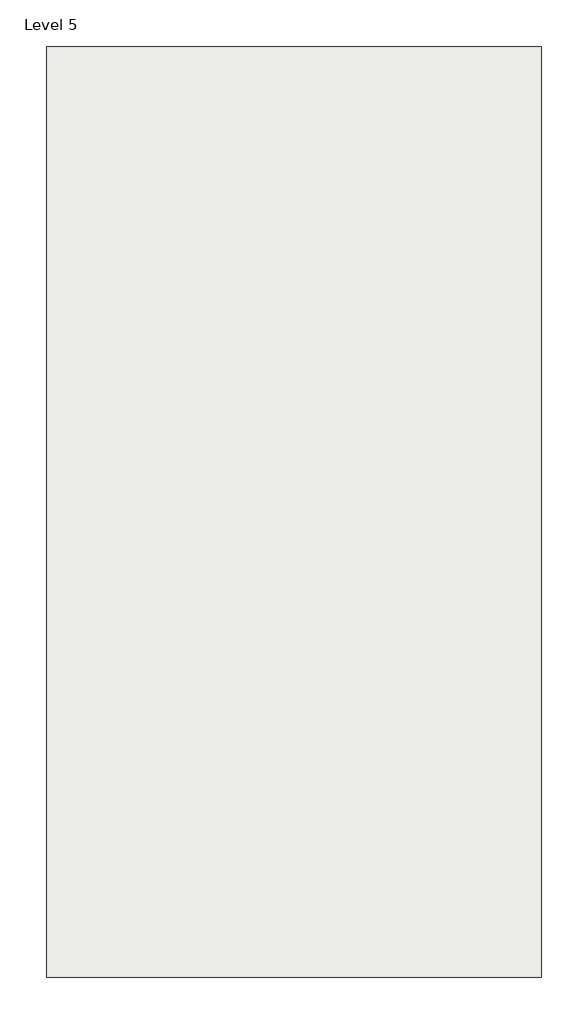
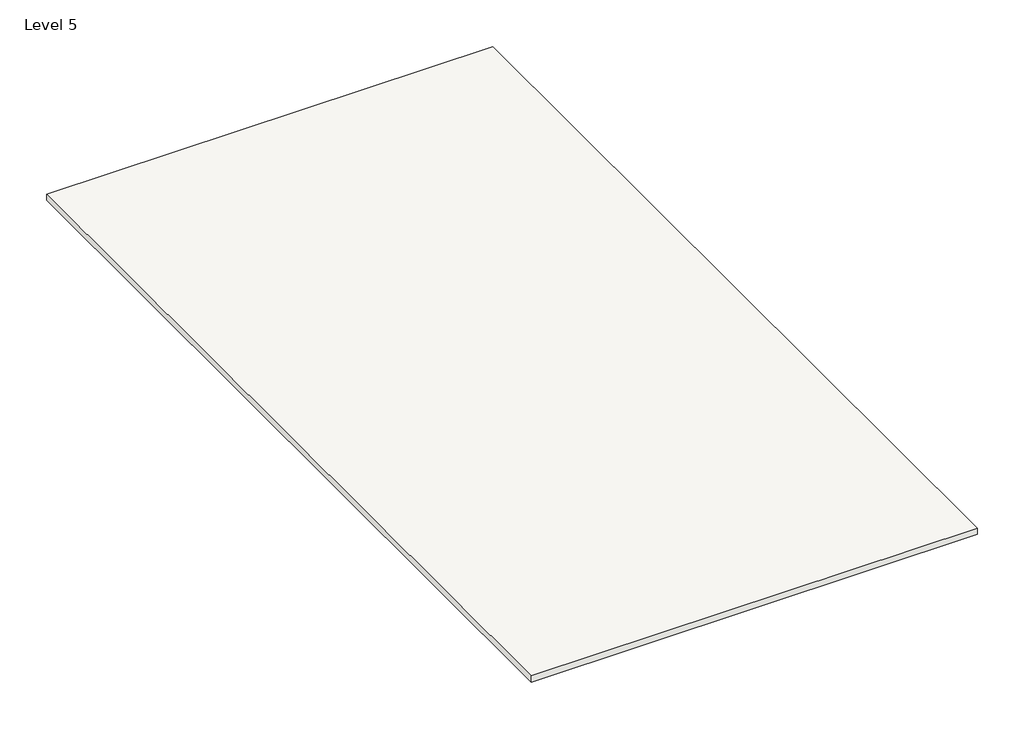
# One storey, incomplete: 1 roof.
"""IFC4 building model written with IfcOpenShell, lengths in millimetres."""

from ifc_helpers import new_model, si_unit, frame, origin, place, context, project, spatial, polyline, outline, extrude, element, save

model = new_model("IFC4")

# Units and contexts
model_context = context("Model", 3, world=origin())
ifc_project = project(units=[si_unit("LENGTHUNIT", "METRE", prefix="MILLI")], contexts=[model_context])

# Site, building, storey
site = spatial("IfcSite", under=ifc_project)
building = spatial("IfcBuilding", under=site)
storey = spatial("IfcBuildingStorey", under=building, Name="Level 5", Elevation=12192.0)

# Roof
placement = place(None, origin())
element("IfcRoof", 1, ObjectType="Generic - 12\"", at=placement, inside=storey, context=model_context, shape_type="SweptSolid", body=[
    extrude(outline(polyline([(660.4, 14579.6), (11023.6, 14579.6), (11023.6, -4927.6), (660.4, -4927.6), (660.4, 14579.6)])), frame((0.0, 0.0, 12192.0), z_axis=(0.0, 0.0, 1.0), x_axis=(1.0, 0.0, 0.0)), (0.0, 0.0, 1.0), 152.4),
])

save(model, "model.ifc")

# Revit data of these elements
# Type "Generic - 12\""
#   Assembly Code = "B1020"
#   Layers, outside or top first: 0' - 6" no material (function 1)
# Element 1 (IfcRoof, "Generic - 12\"")
#   built-in parameter 1001705 = 40.5 (stored number, unit not read)
#   built-in parameter 1001710 = 33615
#   Phase Created = New Construction
#   Materials on its faces: "Clad - White", "Default Roof"
# Materials
#   "Clad - White": class "Wood", colour RGB 242 242 238, transparency 0, Cost = 0
#   "Default Roof": colour RGB 88 101 114, transparency 0, Cost = 0
